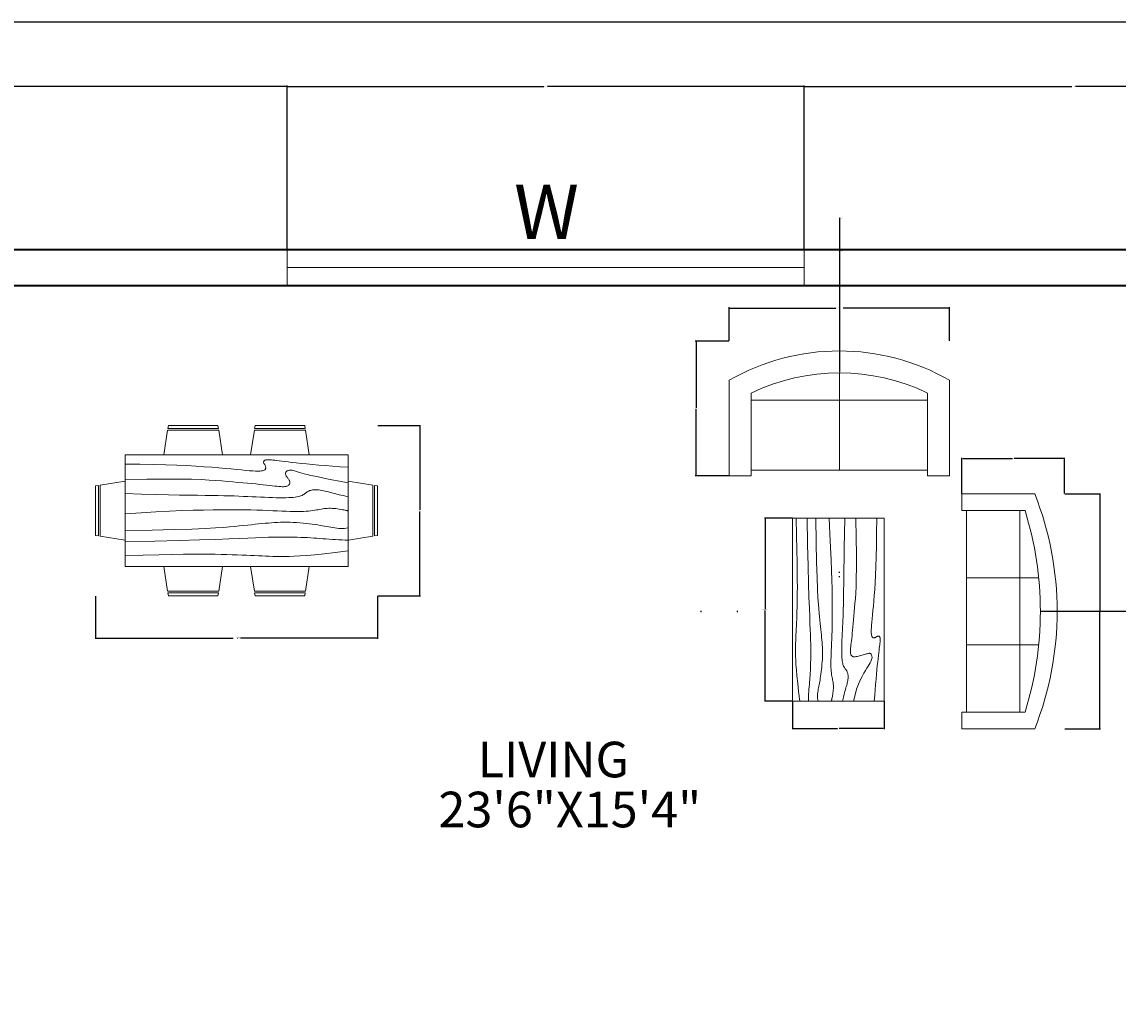
# Model space of a CAD drawing. Units: feet. Extents: x 1755 to 2628, y 1710 to 2329.
# Tile 3 of 4: x 2100 to 2375, y 2081 to 2329. Entities that reach past the tile are written whole.
import ezdxf

# ---------------------------------------------------------------- set-up
doc = ezdxf.new("R2010")
doc.units = ezdxf.units.FT
for name, color, linetype, lineweight in [('A-ANNO-DIMS', 2, 'Continuous', 18), ('A-ANNO-TEXT', 7, 'Continuous', 18), ('A-ANNO-TTLB', 7, 'Continuous', 25), ('A-AREA-IDEN', 7, 'Continuous', 18), ('A-FURN', 8, 'Continuous', 18), ('A-GLAZ', 4, 'Continuous', 18), ('A-WALL', 7, 'Continuous', 35)]:
    doc.layers.add(name, color=color, linetype=linetype, lineweight=lineweight)
doc.styles.get("Standard").update_dxf_attribs({"font": 'arial.ttf'})
doc.dimstyles.get("Standard").update_dxf_attribs({"dimtxt": 0.18, "dimasz": 0.18, "dimexe": 0.18, "dimexo": 0.0625, "dimgap": 0.09, "dimtad": 0, "dimtih": 1, "dimtoh": 1, "dimdec": 4, "dimzin": 0, "dimdsep": 46, "dimtxsty": 'Standard', "dimcen": 0.09, "dimadec": 0, "dimazin": 0, "dimtfac": 1, "dimtdec": 4, "dimtofl": 0, "dimtmove": 0, "dimatfit": 3, "dimfxl": 1, "dimtolj": 1, "dimtzin": 0, "dimarcsym": 0})

# ---------------------------------------------------------------- blocks, each defined once
blk = doc.blocks.new('Sofa - Roundback 7 ft.')
for p, q in [((-12.00002, -32.4421), (-12.00003, -6.5971)), ((11.99997, -32.4421), (11.99998, -6.5971)), ((-36.000027, -34), (-36.000027, -11.4696)), ((35.99998, -34), (35.99998, -11.4696)), ((-35.999844, -13.3819), (35.9998, -13.3819)), ((-36.000027, -32.4421), (35.99998, -32.4421))]:
    blk.add_line(p, q)
for points in [[(-36.000027, -34), (-42.000027, -34), (-42.000027, -8)], [(41.99998, -8), (41.99998, -34), (35.99998, -34)]]:
    blk.add_lwpolyline(points)
for centre, radius, start, end in [((0, -114.25), 114.25, 68.43141, 111.5686), ((-0.00001, -127.1968), 121.1968, 72.72033, 107.2797)]:
    blk.add_arc(centre, radius, start, end)
blk = doc.blocks.new('Sofa - Roundback Loveseat 5 ft.')
for p, q in [((0, -32.44198), (0, -5.99998)), ((-24, -33.99998), (-24, -11.46958)), ((24.00004, -33.99998), (24.00004, -11.46958)), ((-23.9998, -13.38178), (23.99986, -13.38178)), ((-24, -32.44198), (24.00004, -32.44198))]:
    blk.add_line(p, q)
for points in [[(-24, -33.99998), (-30, -33.99998), (-30, -7.99998)], [(30.00004, -7.99998), (30.00004, -33.99998), (24.00004, -33.99998)]]:
    blk.add_lwpolyline(points)
for centre, radius, start, end in [((0, -60.24998), 60.24998, 60.13715, 119.8628), ((0, -61.38438), 55.38444, 64.32083, 115.6792)]:
    blk.add_arc(centre, radius, start, end)
blk = doc.blocks.new('Dining Set - 36 x 72 in.')
for p, q in [((-22.2343, 26.00059), (-23.4847, 17.99762)), ((-22.2304, 26), (-5.7608, 26)), ((-22, 27.5), (-22.1562, 26.50042)), ((-5.8416, 26.5), (-22.1534, 26.5)), ((-22, 27.5), (-6, 27.5)), ((-5.8437, 26.49966), (-6, 27.5)), ((-4.5152, 17.99762), (-5.7655, 25.99926)), ((5.7657, 26.00059), (4.5153, 17.99762)), ((5.7696, 26), (22.2392, 26)), ((6, 27.5), (5.8438, 26.50042)), ((22.1584, 26.5), (5.8466, 26.5)), ((6, 27.5), (22, 27.5)), ((22.1563, 26.49966), (22, 27.5)), ((23.4848, 17.99762), (22.2345, 25.99926)), ((36, 18), (-36, 18)), ((-36, 18), (-36, -18)), ((36, -18), (36, 18)), ((-45.5, 8), (-44.5004, 8.15617)), ((-45.5, 8), (-45.5, -8)), ((-44.5, -8.15843), (-44.5, 8.15338)), ((-44.0006, 8.23428), (-35.9976, 9.48474)), ((-44, 8.23041), (-44, -8.23915)), ((44.0006, 8.23428), (35.9976, 9.48474)), ((44, 8.23041), (44, -8.23915)), ((44.5, -8.15843), (44.5, 8.15338)), ((45.5, 8), (44.5005, 8.15617)), ((45.5, 8), (45.5, -8)), ((-44.4997, -8.15631), (-45.5, -8)), ((-35.9976, -9.48476), (-43.9993, -8.2345)), ((35.9976, -9.48476), (43.9993, -8.2345)), ((44.4997, -8.15631), (45.5, -8)), ((-36, -18), (36, -18)), ((-22.2343, -26.0006), (-23.4847, -17.99762)), ((-4.5152, -17.99762), (-5.7655, -25.99928)), ((5.7657, -26.0006), (4.5153, -17.99762)), ((23.4848, -17.99762), (22.2345, -25.99928)), ((-22.2304, -26), (-5.7608, -26)), ((-22, -27.5), (-22.1562, -26.50044)), ((-5.8416, -26.5), (-22.1534, -26.5)), ((-22, -27.5), (-6, -27.5)), ((-5.8437, -26.49967), (-6, -27.5)), ((5.7696, -26), (22.2392, -26)), ((6, -27.5), (5.8438, -26.50044)), ((22.1584, -26.5), (5.8466, -26.5)), ((6, -27.5), (22, -27.5)), ((22.1563, -26.49967), (22, -27.5))]:
    blk.add_line(p, q)
for points in [[(-36, 15), (-31.1772, 14.97754), (-26.8079, 14.91406), (-22.8538, 14.81543), (-19.276, 14.6875), (-16.0362, 14.53613), (-13.0957, 14.36718), (-10.4159, 14.18652), (-7.9583, 14), (-5.6904, 13.81315), (-3.6035, 13.63021), (-1.6954, 13.45508), (0.0365, 13.29166), (1.5945, 13.14388), (2.9811, 13.01562), (4.1988, 12.9108), (5.25, 12.83333), (6.1393, 12.78613), (6.8802, 12.76823), (7.4883, 12.77767), (7.9792, 12.8125), (8.3685, 12.87077), (8.6719, 12.95052), (8.9049, 13.0498), (9.0833, 13.16666), (9.2205, 13.29899), (9.3216, 13.44401), (9.3895, 13.59879), (9.4271, 13.76041), (9.4373, 13.92594), (9.4232, 14.09245), (9.3875, 14.257), (9.3333, 14.41666), (9.2638, 14.56917), (9.1836, 14.71484), (9.0975, 14.85465), (9.0104, 14.98958), (8.9272, 15.1206), (8.8529, 15.2487), (8.7922, 15.37483), (8.75, 15.5), (8.7305, 15.62467), (8.7344, 15.74739), (8.7617, 15.86621), (8.8125, 15.97916), (8.8867, 16.08431), (8.9844, 16.17968), (9.1055, 16.26334), (9.25, 16.33333), (9.4189, 16.38802), (9.6172, 16.42708), (9.8506, 16.45052), (10.125, 16.45833), (10.4463, 16.45052), (10.8203, 16.42708), (11.2529, 16.38802), (11.75, 16.33333), (12.3184, 16.26318), (12.9694, 16.17838), (13.7151, 16.07991), (14.5677, 15.96875), (15.5395, 15.84586), (16.6426, 15.71224), (17.8893, 15.56884), (19.2917, 15.41666), (20.859, 15.25667), (22.5879, 15.08984), (24.4721, 14.91715), (26.5052, 14.73958), (28.6809, 14.5581), (30.9929, 14.3737), (33.4347, 14.18733), (36, 14)], [(-36, 10), (-28.9766, 10.14274), (-23.1725, 10.20442), (-18.4241, 10.19775), (-14.5677, 10.13541), (-11.4399, 10.03011), (-8.877, 9.89453), (-6.7154, 9.74137), (-4.7917, 9.58333), (-2.9698, 9.43082), (-1.2246, 9.28515), (0.4415, 9.14534), (2.026, 9.01041), (3.5266, 8.87939), (4.9408, 8.7513), (6.266, 8.62516), (7.5, 8.5), (8.6411, 8.37549), (9.6914, 8.2539), (10.6538, 8.13818), (11.5312, 8.03125), (12.3267, 7.93603), (13.043, 7.85547), (13.6831, 7.79248), (14.25, 7.75), (14.7471, 7.7303), (15.1797, 7.73307), (15.5537, 7.75732), (15.875, 7.80208), (16.1494, 7.86637), (16.3828, 7.94922), (16.5811, 8.04964), (16.75, 8.16666), (16.8944, 8.29915), (17.0143, 8.44531), (17.1089, 8.60319), (17.1771, 8.77083), (17.218, 8.94629), (17.2305, 9.1276), (17.2137, 9.31282), (17.1667, 9.5), (17.0895, 9.6875), (16.987, 9.875), (16.8649, 10.0625), (16.7292, 10.25), (16.5856, 10.4375), (16.4401, 10.625), (16.2985, 10.8125), (16.1667, 11), (16.05, 11.18733), (15.9518, 11.3737), (15.8752, 11.5581), (15.8229, 11.73958), (15.798, 11.91715), (15.8034, 12.08984), (15.842, 12.25667), (15.9167, 12.41666), (16.0295, 12.56836), (16.1784, 12.70833), (16.3605, 12.83268), (16.5729, 12.9375), (16.8127, 13.01888), (17.0768, 13.07291), (17.3625, 13.0957), (17.6667, 13.08333), (17.9894, 13.03312), (18.3418, 12.94726), (18.7382, 12.82918), (19.1927, 12.68229), (19.7195, 12.51001), (20.3327, 12.31575), (21.0465, 12.10294), (21.875, 11.875), (22.8357, 11.63354), (23.959, 11.37304), (25.2786, 11.08618), (26.8282, 10.76562), (28.6414, 10.40405), (30.752, 9.99414), (33.1936, 9.52856), (36, 9)], [(-36, 5.5), (-30.7157, 5.3348), (-26.069, 5.20963), (-21.9946, 5.11767), (-18.4271, 5.05208), (-15.3009, 5.00602), (-12.5508, 4.97265), (-10.1112, 4.94515), (-7.9167, 4.91666), (-5.909, 4.88167), (-4.0586, 4.83984), (-2.3429, 4.79215), (-0.7396, 4.73958), (0.7739, 4.6831), (2.22, 4.6237), (3.6213, 4.56233), (5, 4.5), (6.373, 4.43782), (7.7344, 4.3776), (9.0723, 4.32129), (10.375, 4.27083), (11.6309, 4.22819), (12.8281, 4.19531), (13.9551, 4.17415), (15, 4.16666), (15.954, 4.17448), (16.819, 4.19791), (17.6001, 4.23698), (18.3021, 4.29166), (18.9299, 4.36198), (19.4883, 4.44791), (19.9823, 4.54948), (20.4167, 4.66666), (20.7969, 4.79899), (21.1302, 4.94401), (21.4245, 5.09879), (21.6875, 5.26041), (21.9271, 5.42594), (22.1511, 5.59245), (22.3672, 5.757), (22.5834, 5.91666), (22.8065, 6.06868), (23.0404, 6.21093), (23.2879, 6.34147), (23.5521, 6.45833), (23.8358, 6.55957), (24.142, 6.64323), (24.4735, 6.70735), (24.8334, 6.75), (25.2235, 6.76969), (25.642, 6.76692), (26.0858, 6.74267), (26.5521, 6.69791), (27.0379, 6.63362), (27.5404, 6.55078), (28.0565, 6.45036), (28.5834, 6.33333), (29.1242, 6.19987), (29.7071, 6.04687), (30.3661, 5.87044), (31.1354, 5.66666), (32.0493, 5.43164), (33.142, 5.16146), (34.4475, 4.85221), (36, 4.5)], [(-36, -1), (-30.7915, -0.6591), (-26.0195, -0.38216), (-21.6519, -0.16284), (-17.6563, 0.00521), (-14.0005, 0.12833), (-10.6523, 0.21289), (-7.5796, 0.26522), (-4.75, 0.29166), (-2.134, 0.29793), (0.2878, 0.28711), (2.5317, 0.26163), (4.6146, 0.22396), (6.5529, 0.17651), (8.3633, 0.12174), (10.0623, 0.06209), (11.6667, 0), (13.1899, -0.06201), (14.6341, -0.1211), (15.9982, -0.17432), (17.2813, -0.21875), (18.4823, -0.25147), (19.6003, -0.26953), (20.6343, -0.27002), (21.5834, -0.25), (22.4481, -0.20768), (23.2357, -0.14584), (23.9549, -0.06836), (24.6146, 0.02083), (25.2235, 0.11784), (25.7904, 0.21875), (26.3241, 0.31966), (26.8334, 0.41666), (27.3265, 0.50618), (27.8099, 0.58593), (28.2894, 0.65397), (28.7709, 0.70833), (29.2601, 0.74707), (29.763, 0.76823), (30.2855, 0.76985), (30.8334, 0.75), (31.4088, 0.70784), (31.9994, 0.64713), (32.589, 0.57275), (33.1615, 0.48958), (33.7008, 0.4025), (34.1908, 0.3164), (34.6153, 0.23616), (34.9584, 0.16666), (35.2099, 0.11165), (35.3848, 0.07031), (35.504, 0.04069), (35.5886, 0.02083), (35.6594, 0.00879), (35.7377, 0.0026), (35.8442, 0.00032), (36, 0)], [(-36, -6.5), (-27.1843, -6.31267), (-20.084, -6.1263), (-14.469, -5.9419), (-10.1094, -5.76042), (-6.7752, -5.58285), (-4.2363, -5.41016), (-2.2629, -5.24333), (-0.625, -5.08334), (0.8708, -4.93099), (2.2715, -4.78646), (3.5872, -4.64974), (4.8281, -4.52084), (6.0046, -4.39974), (7.127, -4.28646), (8.2053, -4.18099), (9.25, -4.08334), (10.2705, -3.99382), (11.2734, -3.91407), (12.2647, -3.84603), (13.25, -3.79167), (14.2354, -3.75293), (15.2266, -3.73177), (16.2295, -3.73015), (17.25, -3.75), (18.2912, -3.79248), (19.3451, -3.85547), (20.4009, -3.93604), (21.4479, -4.03125), (22.4754, -4.13819), (23.4727, -4.25391), (24.4289, -4.37549), (25.3334, -4.5), (26.1785, -4.62492), (26.9694, -4.74935), (27.7145, -4.87281), (28.4219, -4.99479), (29.1, -5.11483), (29.7572, -5.23242), (30.4016, -5.34709), (31.0417, -5.45834), (31.6837, -5.56437), (32.3262, -5.65821), (32.9658, -5.73153), (33.599, -5.77604), (34.2224, -5.78345), (34.8327, -5.74545), (35.4264, -5.65373), (36, -5.5)], [(-36, -10), (-26.4022, -9.81299), (-18.4675, -9.62891), (-11.9839, -9.45069), (-6.7396, -9.28125), (-2.5226, -9.12354), (0.8789, -8.98047), (3.6769, -8.85498), (6.0833, -8.75), (8.2767, -8.66765), (10.3021, -8.60677), (12.1712, -8.56543), (13.8958, -8.54167), (15.4876, -8.53353), (16.9583, -8.53907), (18.3197, -8.55632), (19.5834, -8.58334), (20.7616, -8.61841), (21.8685, -8.66081), (22.9188, -8.71004), (23.9271, -8.76563), (24.9081, -8.82707), (25.8763, -8.89388), (26.8465, -8.96558), (27.8334, -9.04167), (28.8474, -9.12118), (29.8828, -9.20117), (30.93, -9.27824), (31.9792, -9.34896), (33.0205, -9.40991), (34.0443, -9.45768), (35.0407, -9.48885), (36, -9.5)], [(-36, -14.5), (-30.0881, -14.33513), (-25.0332, -14.21224), (-20.7312, -14.12647), (-17.0781, -14.07292), (-13.97, -14.04671), (-11.3027, -14.04297), (-8.9724, -14.05681), (-6.875, -14.08334), (-4.9224, -14.11833), (-3.0905, -14.16016), (-1.3709, -14.20785), (0.2448, -14.26042), (1.7647, -14.3169), (3.1973, -14.3763), (4.5507, -14.43767), (5.8333, -14.5), (7.0554, -14.5621), (8.235, -14.62175), (9.3922, -14.67652), (10.5469, -14.72396), (11.7192, -14.76164), (12.929, -14.78711), (14.1965, -14.79794), (15.5417, -14.79167), (16.9933, -14.76424), (18.6152, -14.70508), (20.4804, -14.60197), (22.6615, -14.44271), (25.2312, -14.21509), (28.2624, -13.9069), (31.8277, -13.50594), (36, -13)]]:
    blk.add_lwpolyline(points)
blk = doc.blocks.new('Table - Rectangular Woodgrain 60 x 30 in.')
for p, q in [((0, 0), (0, -30)), ((60, 0), (0, 0)), ((60, -30), (60, 0)), ((0, -30), (60, -30))]:
    blk.add_line(p, q)
for points in [[(0, -2.4), (4.8155, -2.418), (9.0302, -2.4688), (12.709, -2.5477), (15.9167, -2.65), (18.7181, -2.7711), (21.1781, -2.9063), (23.3616, -3.0508), (25.3333, -3.2), (27.1477, -3.3495), (28.8172, -3.4958), (30.3437, -3.636), (31.7291, -3.7667), (32.9756, -3.8849), (34.0849, -3.9875), (35.059, -4.0714), (35.9, -4.1334), (36.6114, -4.1711), (37.2041, -4.1854), (37.6906, -4.1779), (38.0833, -4.15), (38.3948, -4.1034), (38.6375, -4.0396), (38.8239, -3.9602), (38.9666, -3.8667), (39.0764, -3.7608), (39.1573, -3.6448), (39.2116, -3.521), (39.2416, -3.3917), (39.2498, -3.2593), (39.2385, -3.1261), (39.21, -2.9944), (39.1666, -2.8667), (39.111, -2.7447), (39.0468, -2.6281), (38.978, -2.5163), (38.9083, -2.4083), (38.8418, -2.3035), (38.7823, -2.201), (38.7337, -2.1001), (38.7, -2), (38.6844, -1.9003), (38.6875, -1.8021), (38.7094, -1.707), (38.75, -1.6167), (38.8094, -1.5326), (38.8875, -1.4563), (38.9844, -1.3893), (39.1, -1.3333), (39.2351, -1.2896), (39.3937, -1.2583), (39.5804, -1.2396), (39.8, -1.2333), (40.057, -1.2396), (40.3562, -1.2583), (40.7023, -1.2896), (41.1, -1.3333), (41.5547, -1.3895), (42.0755, -1.4573), (42.6721, -1.5361), (43.3542, -1.625), (44.1316, -1.7233), (45.014, -1.8302), (46.0114, -1.9449), (47.1333, -2.0667), (48.3862, -2.1947), (49.7625, -2.3281), (51.2513, -2.4663), (52.8416, -2.6083), (54.5226, -2.7535), (56.2833, -2.9011), (58.1127, -3.0501), (60, -3.2)], [(0, -9.2), (6.5759, -9.0858), (11.9385, -9.0365), (16.2527, -9.0418), (19.6833, -9.0917), (22.3952, -9.1759), (24.5531, -9.2844), (26.322, -9.4069), (27.8666, -9.5333), (29.3241, -9.6553), (30.7203, -9.7719), (32.0532, -9.8837), (33.3208, -9.9917), (34.5213, -10.0965), (35.6526, -10.199), (36.7128, -10.2999), (37.7, -10.4), (38.6129, -10.4996), (39.4531, -10.5969), (40.223, -10.6895), (40.925, -10.775), (41.5613, -10.8512), (42.1344, -10.9156), (42.6465, -10.966), (43.1, -11), (43.4976, -11.0158), (43.8437, -11.0136), (44.143, -10.9942), (44.4, -10.9583), (44.6195, -10.9069), (44.8062, -10.8406), (44.9648, -10.7603), (45.1, -10.6667), (45.2155, -10.5598), (45.3114, -10.4365), (45.3871, -10.2929), (45.4416, -10.125), (45.4743, -9.929), (45.4844, -9.7011), (45.4709, -9.4371), (45.4333, -9.1333), (45.3716, -8.7883), (45.2896, -8.4104), (45.1919, -8.0107), (45.0833, -7.6), (44.9685, -7.1893), (44.8521, -6.7896), (44.7388, -6.4117), (44.6333, -6.0667), (44.54, -5.7628), (44.4614, -5.4979), (44.4001, -5.2675), (44.3583, -5.0667), (44.3384, -4.8909), (44.3427, -4.7354), (44.3736, -4.5956), (44.4333, -4.4667), (44.5236, -4.3453), (44.6427, -4.2333), (44.7884, -4.1339), (44.9583, -4.05), (45.1501, -3.9849), (45.3614, -3.9417), (45.59, -3.9234), (45.8333, -3.9333), (46.0915, -3.9749), (46.3734, -4.0531), (46.6906, -4.1736), (47.0542, -4.3417), (47.4756, -4.5629), (47.9661, -4.8427), (48.5372, -5.1866), (49.2, -5.6), (49.9676, -6.0844), (50.8594, -6.625), (51.8965, -7.2031), (53.1, -7.8), (54.491, -8.3969), (56.0906, -8.975), (57.9199, -9.5156), (60, -10)], [(0, -12.8), (5.1847, -12.9322), (9.6213, -13.0323), (13.3963, -13.1059), (16.5958, -13.1583), (19.3063, -13.1952), (21.614, -13.2219), (23.6054, -13.2439), (25.3666, -13.2667), (26.9728, -13.2947), (28.4531, -13.3281), (29.8256, -13.3663), (31.1083, -13.4083), (32.3191, -13.4535), (33.476, -13.501), (34.597, -13.5501), (35.7, -13.6), (36.7984, -13.6497), (37.8875, -13.6979), (38.9578, -13.743), (40, -13.7833), (41.0047, -13.8174), (41.9625, -13.8438), (42.864, -13.8607), (43.7, -13.8667), (44.4631, -13.8604), (45.1552, -13.8417), (45.7801, -13.8104), (46.3416, -13.7667), (46.8439, -13.7104), (47.2906, -13.6417), (47.6858, -13.5604), (48.0333, -13.4667), (48.3375, -13.3608), (48.6042, -13.2448), (48.8396, -13.121), (49.05, -12.9917), (49.2417, -12.8593), (49.4208, -12.7261), (49.5937, -12.5944), (49.7667, -12.4667), (49.9452, -12.3451), (50.1323, -12.2313), (50.3303, -12.1268), (50.5416, -12.0333), (50.7686, -11.9524), (51.0135, -11.8854), (51.2788, -11.8341), (51.5666, -11.8), (51.8785, -11.7843), (52.2116, -11.7865), (52.562, -11.8059), (52.926, -11.8417), (53.2998, -11.8931), (53.6795, -11.9594), (54.0614, -12.0397), (54.4416, -12.1333), (54.8223, -12.2401), (55.2293, -12.3625), (55.6942, -12.5037), (56.2489, -12.6667), (56.9251, -12.8547), (57.7545, -13.0708), (58.7689, -13.3182), (60, -13.6)], [(0, -18), (5.124, -17.7273), (9.6609, -17.5057), (13.6705, -17.3303), (17.2125, -17.1958), (20.3467, -17.0973), (23.1328, -17.0297), (25.6307, -16.9878), (27.9, -16.9667), (29.9928, -16.9617), (31.9302, -16.9703), (33.7254, -16.9907), (35.3917, -17.0208), (36.9423, -17.0588), (38.3906, -17.1026), (39.7499, -17.1503), (41.0333, -17.2), (42.2519, -17.2496), (43.4073, -17.2969), (44.4986, -17.3395), (45.525, -17.375), (46.4858, -17.4012), (47.3802, -17.4156), (48.2074, -17.416), (48.9667, -17.4), (49.6583, -17.3662), (50.2872, -17.3167), (50.8595, -17.2547), (51.3812, -17.1833), (51.8584, -17.1057), (52.2971, -17.025), (52.7034, -16.9443), (53.0833, -16.8667), (53.443, -16.7951), (53.789, -16.7313), (54.128, -16.6768), (54.4666, -16.6334), (54.8115, -16.6024), (55.1693, -16.5854), (55.5465, -16.5841), (55.95, -16.6), (56.3828, -16.6337), (56.8346, -16.6823), (57.2915, -16.7418), (57.7396, -16.8084), (58.165, -16.878), (58.5539, -16.9469), (58.8924, -17.0111), (59.1666, -17.0667), (59.3679, -17.1107), (59.5078, -17.1438), (59.6032, -17.1675), (59.6708, -17.1833), (59.7275, -17.193), (59.7901, -17.1979), (59.8753, -17.1998), (60, -17.2)], [(0, -22.4), (8.0098, -22.2501), (14.4094, -22.1011), (19.4168, -21.9535), (23.25, -21.8083), (26.1269, -21.6663), (28.2656, -21.5281), (29.884, -21.3947), (31.2, -21.2667), (32.3967, -21.1448), (33.5172, -21.0292), (34.5697, -20.9198), (35.5625, -20.8167), (36.5037, -20.7198), (37.4015, -20.6292), (38.2642, -20.5448), (39.1, -20.4667), (39.9164, -20.3951), (40.7187, -20.3313), (41.5117, -20.2768), (42.3, -20.2333), (43.0883, -20.2024), (43.8812, -20.1854), (44.6836, -20.1841), (45.5, -20.2), (46.3328, -20.234), (47.1747, -20.2844), (48.0163, -20.3488), (48.8479, -20.425), (49.66, -20.5106), (50.4429, -20.6031), (51.1872, -20.7004), (51.8833, -20.8), (52.5246, -20.8999), (53.1166, -20.9995), (53.6681, -21.0983), (54.1875, -21.1958), (54.6834, -21.2919), (55.1646, -21.3859), (55.6394, -21.4777), (56.1167, -21.5667), (56.6028, -21.6515), (57.0961, -21.7266), (57.5929, -21.7852), (58.0896, -21.8208), (58.5823, -21.8268), (59.0674, -21.7964), (59.5412, -21.723), (60, -21.6)], [(0, -25.2), (8.6355, -25.0504), (15.7026, -24.9031), (21.4049, -24.7606), (25.9458, -24.625), (29.529, -24.4988), (32.3578, -24.3844), (34.6359, -24.284), (36.5667, -24.2), (38.3213, -24.1341), (39.9417, -24.0854), (41.437, -24.0523), (42.8167, -24.0333), (44.0901, -24.0268), (45.2667, -24.0313), (46.3557, -24.0451), (47.3667, -24.0667), (48.309, -24.0947), (49.1928, -24.1287), (50.0284, -24.168), (50.826, -24.2125), (51.5959, -24.2617), (52.3483, -24.3151), (53.0935, -24.3725), (53.8417, -24.4334), (54.6009, -24.497), (55.3699, -24.561), (56.1454, -24.6226), (56.9239, -24.6792), (57.7021, -24.7279), (58.4764, -24.7662), (59.2435, -24.7911), (60, -24.8)], [(0, -28.8), (5.6867, -28.6681), (10.45, -28.5698), (14.407, -28.5012), (17.675, -28.4584), (20.3711, -28.4374), (22.6125, -28.4344), (24.5164, -28.4455), (26.2, -28.4667), (27.762, -28.4947), (29.2276, -28.5281), (30.6033, -28.5663), (31.8958, -28.6084), (33.1118, -28.6535), (34.2578, -28.7011), (35.3405, -28.7501), (36.3666, -28.8), (37.3443, -28.8497), (38.288, -28.8974), (39.2137, -28.9412), (40.1375, -28.9792), (41.0753, -29.0093), (42.0432, -29.0297), (43.0572, -29.0384), (44.1333, -29.0333), (45.2936, -29.0114), (46.5843, -28.9641), (48.0579, -28.8816), (49.7666, -28.7542), (51.7629, -28.5721), (54.0989, -28.3255), (56.8272, -28.0048), (60, -27.6)]]:
    blk.add_lwpolyline(points)
blk = doc.blocks.new('*D14')
at = {"layer": 'A-ANNO-DIMS', "color": 0, "lineweight": -2, "transparency": 16777216}
for p, q in [((2361.43, 2210.55), (2370.39, 2210.55)), ((2370.21, 2210.37), (2370.21, 2181.26)), ((2370.21, 2151.78), (2370.21, 2180.89)), ((2361.43, 2151.6), (2370.39, 2151.6))]:
    blk.add_line(p, q, dxfattribs=at)
at = {"layer": 'A-ANNO-DIMS', "color": 0, "transparency": 16777216}
for points in [[(2370.18, 2210.37), (2370.24, 2210.37), (2370.21, 2210.55)], [(2370.18, 2151.78), (2370.24, 2151.78), (2370.21, 2151.6)]]:
    blk.add_solid(points, dxfattribs=at)
at = {"layer": 'Defpoints', "color": 0, "transparency": 16777216}
for p in [(2361.36, 2210.55), (2361.36, 2151.6), (2370.21, 2151.6)]:
    blk.add_point(p, dxfattribs=at)
at = {"layer": 'A-ANNO-DIMS', "color": 0, "transparency": 16777216, "insert": (2370.21, 2181.08), "char_height": 0.18, "attachment_point": 5}
blk.add_mtext('\\A1;SOFA 59', dxfattribs=at)
blk = doc.blocks.new('*D15')
at = {"layer": 'A-ANNO-DIMS', "color": 0, "lineweight": -2, "transparency": 16777216}
for p, q in [((2335.63, 2210.61), (2335.63, 2219.57)), ((2335.81, 2219.39), (2348.28, 2219.39)), ((2361.18, 2219.39), (2348.72, 2219.39)), ((2361.36, 2210.61), (2361.36, 2219.57))]:
    blk.add_line(p, q, dxfattribs=at)
at = {"layer": 'A-ANNO-DIMS', "color": 0, "transparency": 16777216}
for points in [[(2335.81, 2219.42), (2335.81, 2219.36), (2335.63, 2219.39)], [(2361.18, 2219.42), (2361.18, 2219.36), (2361.36, 2219.39)]]:
    blk.add_solid(points, dxfattribs=at)
at = {"layer": 'Defpoints', "color": 0, "transparency": 16777216}
for p in [(2361.36, 2219.39), (2335.63, 2210.55), (2361.36, 2210.55)]:
    blk.add_point(p, dxfattribs=at)
at = {"layer": 'A-ANNO-DIMS', "color": 0, "transparency": 16777216, "insert": (2348.5, 2219.39), "char_height": 0.18, "attachment_point": 5}
blk.add_mtext('\\A1;26', dxfattribs=at)
blk = doc.blocks.new('*D16')
at = {"layer": 'A-ANNO-DIMS', "color": 0, "lineweight": -2, "transparency": 16777216}
for p, q in [((2277.24, 2248.93), (2277.24, 2257.35)), ((2277.42, 2257.17), (2303.97, 2257.17)), ((2332.35, 2257.17), (2305.8, 2257.17)), ((2332.53, 2248.93), (2332.53, 2257.35))]:
    blk.add_line(p, q, dxfattribs=at)
at = {"layer": 'A-ANNO-DIMS', "color": 0, "transparency": 16777216}
for points in [[(2277.42, 2257.2), (2277.42, 2257.14), (2277.24, 2257.17)], [(2332.35, 2257.2), (2332.35, 2257.14), (2332.53, 2257.17)]]:
    blk.add_solid(points, dxfattribs=at)
at = {"layer": 'Defpoints', "color": 0, "transparency": 16777216}
for p in [(2332.53, 2257.17), (2277.24, 2248.87), (2332.53, 2248.87)]:
    blk.add_point(p, dxfattribs=at)
at = {"layer": 'A-ANNO-DIMS', "color": 0, "transparency": 16777216, "insert": (2304.88, 2257.17), "char_height": 0.18, "attachment_point": 5}
blk.add_mtext('\\A1;LOVESEAT 55', dxfattribs=at)
blk = doc.blocks.new('*D17')
at = {"layer": 'A-ANNO-DIMS', "color": 0, "lineweight": -2, "transparency": 16777216}
for p, q in [((2277.17, 2248.87), (2268.76, 2248.87)), ((2268.94, 2248.69), (2268.94, 2232.16)), ((2268.94, 2215.26), (2268.94, 2231.79)), ((2277.17, 2215.08), (2268.76, 2215.08))]:
    blk.add_line(p, q, dxfattribs=at)
at = {"layer": 'A-ANNO-DIMS', "color": 0, "transparency": 16777216}
for points in [[(2268.91, 2248.69), (2268.97, 2248.69), (2268.94, 2248.87)], [(2268.91, 2215.26), (2268.97, 2215.26), (2268.94, 2215.08)]]:
    blk.add_solid(points, dxfattribs=at)
at = {"layer": 'Defpoints', "color": 0, "transparency": 16777216}
for p in [(2268.94, 2248.87), (2277.24, 2248.87), (2277.24, 2215.08)]:
    blk.add_point(p, dxfattribs=at)
at = {"layer": 'A-ANNO-DIMS', "color": 0, "transparency": 16777216, "insert": (2268.94, 2231.97), "char_height": 0.18, "attachment_point": 5}
blk.add_mtext('\\A1;34', dxfattribs=at)
blk = doc.blocks.new('*D18')
at = {"layer": 'A-ANNO-DIMS', "color": 0, "lineweight": -2, "transparency": 16777216}
for p, q in [((2118.36, 2184.9), (2118.36, 2174.18)), ((2189.07, 2184.9), (2189.07, 2174.18)), ((2118.54, 2174.36), (2152.76, 2174.36)), ((2188.89, 2174.36), (2154.67, 2174.36))]:
    blk.add_line(p, q, dxfattribs=at)
at = {"layer": 'A-ANNO-DIMS', "color": 0, "transparency": 16777216}
for points in [[(2118.54, 2174.39), (2118.54, 2174.33), (2118.36, 2174.36)], [(2188.89, 2174.39), (2188.89, 2174.33), (2189.07, 2174.36)]]:
    blk.add_solid(points, dxfattribs=at)
at = {"layer": 'Defpoints', "color": 0, "transparency": 16777216}
for p in [(2118.36, 2184.97), (2189.07, 2184.97), (2189.07, 2174.36)]:
    blk.add_point(p, dxfattribs=at)
at = {"layer": 'A-ANNO-DIMS', "color": 0, "transparency": 16777216, "insert": (2153.71, 2174.36), "char_height": 0.18, "attachment_point": 5}
blk.add_mtext('\\A1;DINING SET 71', dxfattribs=at)
blk = doc.blocks.new('*D19')
at = {"layer": 'A-ANNO-DIMS', "color": 0, "lineweight": -2, "transparency": 16777216}
for p, q in [((2189.13, 2227.7), (2199.86, 2227.7)), ((2199.68, 2227.52), (2199.68, 2206.52)), ((2199.68, 2185.15), (2199.68, 2206.15)), ((2189.13, 2184.97), (2199.86, 2184.97))]:
    blk.add_line(p, q, dxfattribs=at)
at = {"layer": 'A-ANNO-DIMS', "color": 0, "transparency": 16777216}
for points in [[(2199.65, 2227.52), (2199.71, 2227.52), (2199.68, 2227.7)], [(2199.65, 2185.15), (2199.71, 2185.15), (2199.68, 2184.97)]]:
    blk.add_solid(points, dxfattribs=at)
at = {"layer": 'Defpoints', "color": 0, "transparency": 16777216}
for p in [(2189.07, 2227.7), (2199.68, 2227.7), (2189.07, 2184.97)]:
    blk.add_point(p, dxfattribs=at)
at = {"layer": 'A-ANNO-DIMS', "color": 0, "transparency": 16777216, "insert": (2199.68, 2206.34), "char_height": 0.18, "attachment_point": 5}
blk.add_mtext('\\A1;43', dxfattribs=at)
blk = doc.blocks.new('*D20')
at = {"layer": 'A-ANNO-DIMS', "color": 0, "lineweight": -2, "transparency": 16777216}
for p, q in [((2293.09, 2204.45), (2286.09, 2204.45)), ((2286.27, 2204.27), (2286.27, 2181.7)), ((2286.27, 2158.77), (2286.27, 2181.33)), ((2293.09, 2158.59), (2286.09, 2158.59))]:
    blk.add_line(p, q, dxfattribs=at)
at = {"layer": 'A-ANNO-DIMS', "color": 0, "transparency": 16777216}
for points in [[(2286.24, 2204.27), (2286.3, 2204.27), (2286.27, 2204.45)], [(2286.24, 2158.77), (2286.3, 2158.77), (2286.27, 2158.59)]]:
    blk.add_solid(points, dxfattribs=at)
at = {"layer": 'Defpoints', "color": 0, "transparency": 16777216}
for p in [(2293.15, 2204.45), (2286.27, 2158.59), (2293.15, 2158.59)]:
    blk.add_point(p, dxfattribs=at)
at = {"layer": 'A-ANNO-DIMS', "color": 0, "transparency": 16777216, "insert": (2286.27, 2181.52), "char_height": 0.18, "attachment_point": 5}
blk.add_mtext('\\A1;LOW TABLE 46', dxfattribs=at)
blk = doc.blocks.new('*D21')
at = {"layer": 'A-ANNO-DIMS', "color": 0, "lineweight": -2, "transparency": 16777216}
for p, q in [((2293.15, 2158.52), (2293.15, 2151.53)), ((2316.08, 2158.52), (2316.08, 2151.53)), ((2293.33, 2151.71), (2304.39, 2151.71)), ((2315.9, 2151.71), (2304.83, 2151.71))]:
    blk.add_line(p, q, dxfattribs=at)
at = {"layer": 'A-ANNO-DIMS', "color": 0, "transparency": 16777216}
for points in [[(2293.33, 2151.74), (2293.33, 2151.68), (2293.15, 2151.71)], [(2315.9, 2151.74), (2315.9, 2151.68), (2316.08, 2151.71)]]:
    blk.add_solid(points, dxfattribs=at)
at = {"layer": 'Defpoints', "color": 0, "transparency": 16777216}
for p in [(2293.15, 2158.59), (2316.08, 2158.59), (2316.08, 2151.71)]:
    blk.add_point(p, dxfattribs=at)
at = {"layer": 'A-ANNO-DIMS', "color": 0, "transparency": 16777216, "insert": (2304.61, 2151.71), "char_height": 0.18, "attachment_point": 5}
blk.add_mtext('\\A1;23', dxfattribs=at)
blk = doc.blocks.new('*D26')
at = {"layer": 'A-ANNO-DIMS', "color": 0, "lineweight": -2, "transparency": 16777216}
for p, q in [((1905.69, 2271.88), (1905.69, 2312.95)), ((1905.87, 2312.77), (2035.59, 2312.77)), ((2166.25, 2312.77), (2036.53, 2312.77)), ((2166.43, 2271.88), (2166.43, 2312.95))]:
    blk.add_line(p, q, dxfattribs=at)
at = {"layer": 'A-ANNO-DIMS', "color": 0, "transparency": 16777216}
for points in [[(1905.87, 2312.8), (1905.87, 2312.74), (1905.69, 2312.77)], [(2166.25, 2312.8), (2166.25, 2312.74), (2166.43, 2312.77)]]:
    blk.add_solid(points, dxfattribs=at)
at = {"layer": 'Defpoints', "color": 0, "transparency": 16777216}
for p in [(2166.43, 2312.77), (1905.69, 2271.82), (2166.43, 2271.82)]:
    blk.add_point(p, dxfattribs=at)
at = {"layer": 'A-ANNO-DIMS', "color": 0, "transparency": 16777216, "insert": (2036.06, 2312.77), "char_height": 0.18, "attachment_point": 5}
blk.add_mtext('\\A1;260.75', dxfattribs=at)
blk = doc.blocks.new('*D27')
at = {"layer": 'A-ANNO-DIMS', "color": 0, "lineweight": -2, "transparency": 16777216}
for p, q in [((2166.43, 2271.88), (2166.43, 2312.95)), ((2166.61, 2312.77), (2230.79, 2312.77)), ((2295.88, 2312.77), (2231.7, 2312.77)), ((2296.06, 2271.88), (2296.06, 2312.95))]:
    blk.add_line(p, q, dxfattribs=at)
at = {"layer": 'A-ANNO-DIMS', "color": 0, "transparency": 16777216}
for points in [[(2166.61, 2312.8), (2166.61, 2312.74), (2166.43, 2312.77)], [(2295.88, 2312.8), (2295.88, 2312.74), (2296.06, 2312.77)]]:
    blk.add_solid(points, dxfattribs=at)
at = {"layer": 'Defpoints', "color": 0, "transparency": 16777216}
for p in [(2296.06, 2312.77), (2166.43, 2271.82), (2296.06, 2271.82)]:
    blk.add_point(p, dxfattribs=at)
at = {"layer": 'A-ANNO-DIMS', "color": 0, "transparency": 16777216, "insert": (2231.25, 2312.77), "char_height": 0.18, "attachment_point": 5}
blk.add_mtext('\\A1;129.63', dxfattribs=at)
blk = doc.blocks.new('*D28')
at = {"layer": 'A-ANNO-DIMS', "color": 0, "lineweight": -2, "transparency": 16777216}
for p, q in [((2296.06, 2271.88), (2296.06, 2312.95)), ((2296.24, 2312.77), (2363.18, 2312.77)), ((2431.02, 2312.77), (2364.09, 2312.77)), ((2431.2, 2271.88), (2431.2, 2312.95))]:
    blk.add_line(p, q, dxfattribs=at)
at = {"layer": 'A-ANNO-DIMS', "color": 0, "transparency": 16777216}
for points in [[(2296.24, 2312.8), (2296.24, 2312.74), (2296.06, 2312.77)], [(2431.02, 2312.8), (2431.02, 2312.74), (2431.2, 2312.77)]]:
    blk.add_solid(points, dxfattribs=at)
at = {"layer": 'Defpoints', "color": 0, "transparency": 16777216}
for p in [(2431.2, 2312.77), (2296.06, 2271.82), (2431.2, 2271.82)]:
    blk.add_point(p, dxfattribs=at)
at = {"layer": 'A-ANNO-DIMS', "color": 0, "transparency": 16777216, "insert": (2363.63, 2312.77), "char_height": 0.18, "attachment_point": 5}
blk.add_mtext('\\A1;135.14', dxfattribs=at)
blk = doc.blocks.new('*D55')
at = {"layer": 'A-ANNO-DIMS', "color": 0, "lineweight": -2, "transparency": 16777216}
for p, q in [((2270.14, 2181.08), (2270.32, 2181.08)), ((2270.23, 2180.99), (2270.23, 2181.17)), ((2406.31, 2181.08), (2355.46, 2181.08))]:
    blk.add_line(p, q, dxfattribs=at)
at = {"layer": 'A-ANNO-DIMS', "color": 0, "transparency": 16777216}
blk.add_solid([(2355.46, 2181.11), (2355.46, 2181.05), (2355.28, 2181.08)], dxfattribs=at)
at = {"layer": 'Defpoints', "color": 0, "transparency": 16777216}
for p in [(2270.23, 2181.08), (2355.28, 2181.08)]:
    blk.add_point(p, dxfattribs=at)
at = {"layer": 'A-ANNO-DIMS', "color": 0, "transparency": 16777216, "insert": (2406.79, 2181.08), "char_height": 0.18, "attachment_point": 5}
blk.add_mtext('\\A1;R85.05', dxfattribs=at)
blk = doc.blocks.new('*D56')
at = {"layer": 'A-ANNO-DIMS', "color": 0, "lineweight": -2, "transparency": 16777216}
for p, q in [((2279.23, 2181.08), (2279.41, 2181.08)), ((2279.32, 2180.99), (2279.32, 2181.17)), ((2407.6, 2181.08), (2359.67, 2181.08))]:
    blk.add_line(p, q, dxfattribs=at)
at = {"layer": 'A-ANNO-DIMS', "color": 0, "transparency": 16777216}
blk.add_solid([(2359.67, 2181.11), (2359.67, 2181.05), (2359.49, 2181.08)], dxfattribs=at)
at = {"layer": 'Defpoints', "color": 0, "transparency": 16777216}
for p in [(2279.32, 2181.08), (2359.49, 2181.08)]:
    blk.add_point(p, dxfattribs=at)
at = {"layer": 'A-ANNO-DIMS', "color": 0, "transparency": 16777216, "insert": (2408.08, 2181.08), "char_height": 0.18, "attachment_point": 5}
blk.add_mtext('\\A1;R80.17', dxfattribs=at)
blk = doc.blocks.new('*D57')
at = {"layer": 'A-ANNO-DIMS', "color": 0, "lineweight": -2, "transparency": 16777216}
for p, q in [((2305.07, 2279.73), (2304.89, 2279.73)), ((2304.89, 2279.73), (2304.89, 2246.59)), ((2304.79, 2190.88), (2304.97, 2190.88)), ((2304.88, 2190.79), (2304.88, 2190.97))]:
    blk.add_line(p, q, dxfattribs=at)
at = {"layer": 'A-ANNO-DIMS', "color": 0, "transparency": 16777216}
blk.add_solid([(2304.86, 2246.59), (2304.92, 2246.59), (2304.89, 2246.41)], dxfattribs=at)
at = {"layer": 'Defpoints', "color": 0, "transparency": 16777216}
for p in [(2304.89, 2246.41), (2304.88, 2190.88)]:
    blk.add_point(p, dxfattribs=at)
at = {"layer": 'A-ANNO-DIMS', "color": 0, "transparency": 16777216, "insert": (2305.54, 2279.73), "char_height": 0.18, "attachment_point": 5}
blk.add_mtext('\\A1;R55.53', dxfattribs=at)
blk = doc.blocks.new('*D58')
at = {"layer": 'A-ANNO-DIMS', "color": 0, "lineweight": -2, "transparency": 16777216}
for p, q in [((2305.07, 2271.51), (2304.89, 2271.51)), ((2304.89, 2271.51), (2304.89, 2241.06)), ((2304.79, 2189.84), (2304.97, 2189.84)), ((2304.88, 2189.75), (2304.88, 2189.93))]:
    blk.add_line(p, q, dxfattribs=at)
at = {"layer": 'A-ANNO-DIMS', "color": 0, "transparency": 16777216}
blk.add_solid([(2304.86, 2241.06), (2304.92, 2241.06), (2304.89, 2240.88)], dxfattribs=at)
at = {"layer": 'Defpoints', "color": 0, "transparency": 16777216}
for p in [(2304.89, 2240.88), (2304.88, 2189.84)]:
    blk.add_point(p, dxfattribs=at)
at = {"layer": 'A-ANNO-DIMS', "color": 0, "transparency": 16777216, "insert": (2305.54, 2271.51), "char_height": 0.18, "attachment_point": 5}
blk.add_mtext('\\A1;R51.04', dxfattribs=at)

msp = doc.modelspace()

# ---------------------------------------------------------------- linework, layer by layer
at = {"layer": 'A-ANNO-TTLB'}
msp.add_lwpolyline([(1754.8706, 2328.9307), (2627.7013, 2328.9307), (2627.7013, 1709.9251), (1754.8706, 1709.9251)], close=True, dxfattribs=at)
at = {"layer": 'A-GLAZ'}
for p, q in [((2166.4346, 2271.8157), (2166.4346, 2262.8157)), ((2296.063, 2271.8157), (2296.063, 2262.8157)), ((2166.4346, 2267.3157), (2296.063, 2267.3157))]:
    msp.add_line(p, q, dxfattribs=at)
at = {"layer": 'A-WALL'}
for p, q in [((2096.8905, 2271.8157), (2548.8905, 2271.8157)), ((2096.8905, 2262.8157), (2378.8905, 2262.8157))]:
    msp.add_line(p, q, dxfattribs=at)

# ---------------------------------------------------------------- block references
at = {"layer": 'A-FURN'}
for name, p, xscale, yscale, zscale in [('Sofa - Roundback Loveseat 5 ft.', (2304.8848, 2246.4131), 0.9216381896866129, 0.9216381896866129, 0.9216381896866129), ('Dining Set - 36 x 72 in.', (2153.7138, 2206.336), 0.7770396752203605, 0.7770396752203605, 0.7770396752203605)]:
    msp.add_blockref(name, p, dxfattribs=dict(at, xscale=xscale, yscale=yscale, zscale=zscale))
at = {"layer": 'A-FURN', "rotation": 270}
for name, p, xscale, yscale, zscale in [('Sofa - Roundback 7 ft.', (2359.4929, 2181.0761), 0.701739537527213, 0.701739537527213, 0.701739537527213), ('Table - Rectangular Woodgrain 60 x 30 in.', (2316.078, 2204.4465), 0.7643266277093668, 0.7643266277093668, 0.7643266277093668)]:
    msp.add_blockref(name, p, dxfattribs=dict(at, xscale=xscale, yscale=yscale, zscale=zscale))

# ---------------------------------------------------------------- texts
at = {"layer": 'A-ANNO-TEXT'}
msp.add_text('W', height=13.589, dxfattribs=at).set_placement((2223.306, 2274.5049))
at = {"layer": 'A-AREA-IDEN'}
for s, height, p in [('LIVING', 8.93153, (2214.1685, 2139.4499)), ('23\'6"X15\'4"', 8.931529, (2204.3433, 2126.9126))]:
    msp.add_text(s, height=height, dxfattribs=at).set_placement(p)

# ---------------------------------------------------------------- dimensions: what is measured, and where the dimension line sits
at = {"layer": 'A-ANNO-DIMS'}
for base, p1, p2, override, picture, middle in [((2166.4346, 2312.7657), (1905.6851, 2271.8157), (2166.4346, 2271.8157), {"dimdec": 2, "dimlfac": 1, "dimrnd": 0, "dimzin": 0, "dimdsep": 46, "dimlunit": 2}, '*D26', (2036.0599, 2312.7657)), ((2296.063, 2312.7657), (2166.4346, 2271.8157), (2296.063, 2271.8157), {"dimdec": 2, "dimlfac": 1, "dimrnd": 0, "dimzin": 0, "dimdsep": 46, "dimlunit": 2}, '*D27', (2231.2488, 2312.7657)), ((2431.1999, 2312.7657), (2296.063, 2271.8157), (2431.1999, 2271.8157), {"dimdec": 2, "dimlfac": 1, "dimrnd": 0, "dimzin": 0, "dimdsep": 46, "dimlunit": 2}, '*D28', (2363.6315, 2312.7657)), ((2361.3642, 2219.3911), (2335.6338, 2210.5492), (2361.3642, 2210.5492), {"dimdec": 0, "dimlfac": 1, "dimrnd": 0, "dimzin": 0, "dimdsep": 46, "dimlunit": 2}, '*D15', (2348.499, 2219.3911)), ((2316.078, 2151.708), (2293.1482, 2158.5869), (2316.078, 2158.5869), {"dimdec": 0, "dimlfac": 1, "dimrnd": 0, "dimzin": 0, "dimdsep": 46, "dimlunit": 2}, '*D21', (2304.6131, 2151.708))]:
    dim = msp.add_linear_dim(base=base, p1=p1, p2=p2, dimstyle='Standard', override=override, dxfattribs=at)
    dim.commit()
    dim.dimension.update_dxf_attribs({"geometry": picture, "text_midpoint": middle})
for center, mpoint, picture, middle in [((2304.8848, 2190.8844), (2304.885, 2246.4131), '*D57', (2305.545, 2279.7303)), ((2304.8848, 2189.8389), (2304.885, 2240.8833), '*D58', (2305.5446, 2271.51)), ((2270.2339, 2181.0761), (2355.2825, 2181.076), '*D55', (2406.3116, 2181.0759)), ((2279.3192, 2181.0761), (2359.4929, 2181.076), '*D56', (2407.5972, 2181.076))]:
    dim = msp.add_radius_dim(center=center, mpoint=mpoint, dimstyle='Standard', override={"dimdec": 2, "dimlfac": 1, "dimrnd": 0, "dimzin": 0, "dimdsep": 46, "dimlunit": 2}, dxfattribs=at)
    dim.commit()
    dim.dimension.update_dxf_attribs({"geometry": picture, "text_midpoint": middle, "dimtype": 164})
for base, p1, p2, text, picture, middle in [((2332.534, 2257.1656), (2277.2357, 2248.8708), (2332.534, 2248.8708), 'LOVESEAT <>', '*D16', (2304.8848, 2257.1656)), ((2189.0691, 2174.3608), (2118.3584, 2184.9674), (2189.0691, 2184.9674), 'DINING SET <>', '*D18', (2153.7138, 2174.3608))]:
    dim = msp.add_linear_dim(base=base, p1=p1, p2=p2, text=text, dimstyle='Standard', override={"dimdec": 0, "dimlfac": 1, "dimrnd": 0, "dimzin": 0, "dimdsep": 46, "dimlunit": 2}, dxfattribs=at)
    dim.commit()
    dim.dimension.update_dxf_attribs({"geometry": picture, "text_midpoint": middle})
for base, p1, p2, picture, middle in [((2268.9409, 2248.8708), (2277.2357, 2215.0774), (2277.2357, 2248.8708), '*D17', (2268.9409, 2231.9741)), ((2199.6756, 2227.7045), (2189.0691, 2184.9674), (2189.0691, 2227.7045), '*D19', (2199.6756, 2206.336))]:
    dim = msp.add_linear_dim(base=base, p1=p1, p2=p2, angle=90, dimstyle='Standard', override={"dimdec": 0, "dimlfac": 1, "dimrnd": 0, "dimzin": 0, "dimdsep": 46, "dimlunit": 2}, dxfattribs=at)
    dim.commit()
    dim.dimension.update_dxf_attribs({"geometry": picture, "text_midpoint": middle})
for base, p1, p2, text, picture, middle in [((2370.2061, 2151.603), (2361.3642, 2210.5492), (2361.3642, 2151.603), 'SOFA <>', '*D14', (2370.2061, 2181.0761)), ((2286.2693, 2158.5869), (2293.1482, 2204.4465), (2293.1482, 2158.5869), 'LOW TABLE <>', '*D20', (2286.2693, 2181.5167))]:
    dim = msp.add_linear_dim(base=base, p1=p1, p2=p2, angle=270, text=text, dimstyle='Standard', override={"dimdec": 0, "dimlfac": 1, "dimrnd": 0, "dimzin": 0, "dimdsep": 46, "dimlunit": 2}, dxfattribs=at)
    dim.commit()
    dim.dimension.update_dxf_attribs({"geometry": picture, "text_midpoint": middle})

doc.saveas('drawing.dxf')
